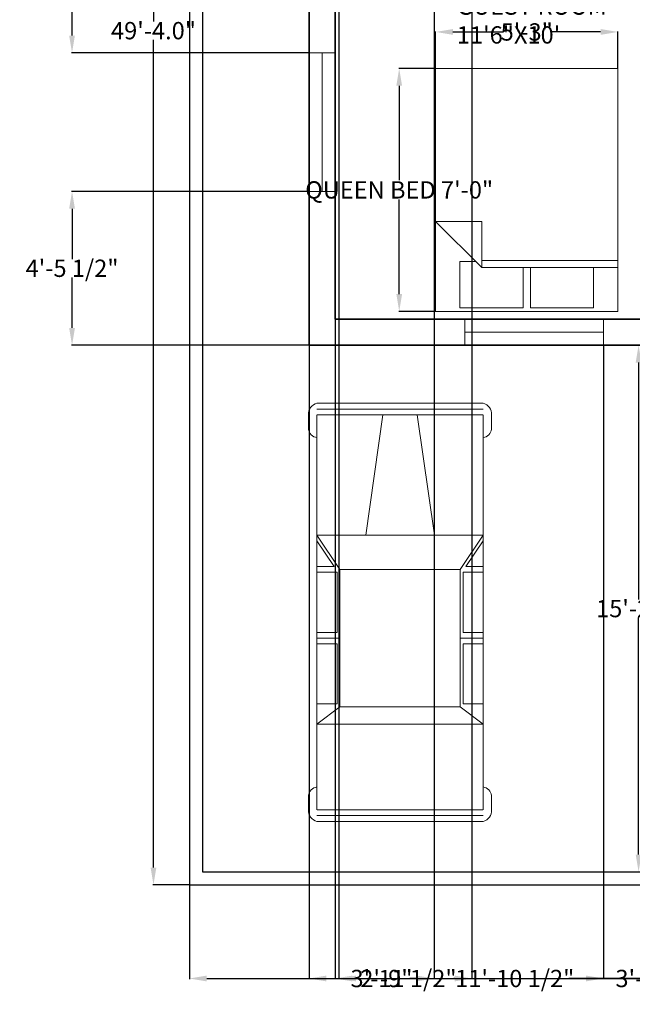
# Model space of a CAD drawing. Units: inches. Extents: x 889 to 1449, y 3224 to 3899.
# Tile 1 of 4: x 889 to 1101, y 3224 to 3565. Entities that reach past the tile are written whole.
import ezdxf

# ---------------------------------------------------------------- set-up
doc = ezdxf.new("R2010")
doc.units = ezdxf.units.IN
doc.header["$MEASUREMENT"] = 0
for name, color, linetype, lineweight in [('A-ANNO-DIMS', 2, 'Continuous', 18), ('A-AREA-IDEN', 7, 'Continuous', 18), ('A-FURN', 8, 'Continuous', 18), ('A-GLAZ', 4, 'Continuous', 18), ('A-WALL', 7, 'Continuous', 35), ('C-PROP', 7, 'Continuous', 25), ('C-SITE-VEHC', 8, 'Continuous', 18)]:
    doc.layers.add(name, color=color, linetype=linetype, lineweight=lineweight)
doc.styles.get("Standard").update_dxf_attribs({"font": 'arial.ttf'})
doc.dimstyles.get("Standard").update_dxf_attribs({"dimtxt": 6, "dimasz": 6, "dimexe": 0.18, "dimexo": 0.0625, "dimgap": 0.09, "dimtad": 0, "dimtih": 1, "dimtoh": 1, "dimdec": 1, "dimzin": 0, "dimdsep": 46, "dimlunit": 3, "dimtxsty": 'Standard', "dimcen": 0.09, "dimadec": 0, "dimazin": 0, "dimtfac": 1, "dimtdec": 1, "dimtofl": 0, "dimtmove": 0, "dimatfit": 3, "dimfxl": 1, "dimtolj": 1, "dimtzin": 0, "dimarcsym": 0})

# ---------------------------------------------------------------- blocks, each defined once
blk = doc.blocks.new('*U13')
for p, q in [((5.44, 42.31), (12.12, 42.31)), ((189.69, 42.31), (183.01, 42.31)), ((0.1, -0.41), (0.1, 38.35)), ((2.77, -0.41), (2.77, 38.31)), ((5.44, -0.41), (5.44, 38.24)), ((5.45, 38.31), (16.12, 38.31)), ((16.12, 38.31), (180.34, 38.31)), ((61.52, -0.41), (61.52, 38.31)), ((61.52, 38.31), (77.54, 27.62)), ((64.19, 38.31), (76.2, 30.29)), ((76.2, 30.29), (76.2, 38.31)), ((78.87, 38.31), (78.87, 28.96)), ((106.91, 28.96), (106.91, 38.31)), ((109.58, 27.62), (109.58, 38.31)), ((112.25, 38.31), (112.25, 28.96)), ((140.29, 28.96), (140.29, 38.31)), ((141.62, 27.62), (149.64, 38.31)), ((149.64, -0.41), (149.64, 38.31)), ((189.69, 38.31), (179.01, 38.31)), ((189.69, -0.41), (189.69, 38.24)), ((192.36, -0.41), (192.36, 38.31)), ((195.03, -0.41), (195.03, 38.35)), ((77.54, 27.62), (141.62, 27.62)), ((77.54, -0.41), (77.54, 27.62)), ((78.87, 28.96), (106.91, 28.96)), ((112.25, 28.96), (140.29, 28.96)), ((141.62, -0.41), (141.62, 27.62)), ((5.44, 7.6), (61.52, 15.61)), ((0.1, -0.42), (0.1, -39.18)), ((2.77, -0.41), (2.77, -39.13)), ((5.44, -0.42), (5.44, -39.07)), ((61.52, -0.41), (61.52, -39.13)), ((77.54, -0.41), (77.54, -28.45)), ((141.62, -0.41), (141.62, -28.45)), ((149.64, -0.41), (149.64, -39.13)), ((189.69, -0.42), (189.69, -39.07)), ((192.36, -0.41), (192.36, -39.13)), ((195.03, -0.42), (195.03, -39.18)), ((5.44, -8.42), (61.52, -16.43)), ((61.52, -39.13), (77.54, -28.45)), ((64.19, -39.13), (76.2, -31.12)), ((76.2, -31.12), (76.2, -39.13)), ((77.54, -28.45), (141.62, -28.45)), ((78.87, -39.13), (78.87, -29.79)), ((78.87, -29.79), (106.91, -29.79)), ((106.91, -29.79), (106.91, -39.13)), ((109.58, -28.45), (109.58, -39.13)), ((112.25, -29.79), (140.29, -29.79)), ((112.25, -39.13), (112.25, -29.79)), ((140.29, -29.79), (140.29, -39.13)), ((141.62, -28.45), (149.64, -39.13)), ((5.45, -39.13), (16.12, -39.13)), ((16.12, -39.13), (180.34, -39.13)), ((189.69, -39.13), (179.01, -39.13)), ((5.44, -43.14), (12.12, -43.14)), ((189.69, -43.14), (183.01, -43.14))]:
    blk.add_line(p, q)
for centre, radius, start, end in [((5.06, 37.26), 5.06, 85.6455, 168.0943), ((11.45, 37.64), 4.72, 8.1301, 81.87), ((183.68, 37.64), 4.72, 98.13, 171.8699), ((190.07, 37.26), 5.06, 11.9057, 94.3545), ((5.06, -38.09), 5.06, 191.9057, 274.3545), ((11.45, -38.46), 4.72, 278.13, 351.8699), ((183.68, -38.46), 4.72, 188.1301, 261.87), ((190.07, -38.09), 5.06, 265.6455, 348.0943)]:
    blk.add_arc(centre, radius, start, end)
blk = doc.blocks.new('Bed - Queen')
for p, q in [((0, -80.00003), (0, 0)), ((0, 0), (59.99999, 0)), ((59.99999, 0), (59.99999, -80.00003)), ((7.99999, -1.2), (28.79998, -1.2)), ((7.99999, -14.4), (7.99999, -1.2)), ((28.79998, -1.2), (28.79998, -14.4)), ((31.19999, -1.2), (51.99999, -1.2)), ((31.19999, -14.4), (31.19999, -1.2)), ((51.99999, -1.2), (51.99999, -16.4)), ((0, -14.4), (44.8, -14.4)), ((59.99999, -29.6), (44.8, -14.4)), ((44.8, -14.4), (44.8, -29.6)), ((44.8, -16.8), (0, -16.8)), ((51.99999, -16.4), (46.79936, -16.4)), ((44.8, -29.6), (59.99999, -29.6)), ((59.99999, -80.00003), (0, -80.00003))]:
    blk.add_line(p, q)
blk = doc.blocks.new('*D19')
at = {"layer": 'A-ANNO-DIMS', "color": 0, "lineweight": -2, "transparency": 16777216}
for p, q in [((947.88, 3857.35), (935.33, 3857.35)), ((935.51, 3851.35), (935.51, 3564.51)), ((935.51, 3271.35), (935.51, 3558.2)), ((947.88, 3265.35), (935.33, 3265.35))]:
    blk.add_line(p, q, dxfattribs=at)
at = {"layer": 'A-ANNO-DIMS', "color": 0, "transparency": 16777216}
for points in [[(934.51, 3851.35), (936.51, 3851.35), (935.51, 3857.35)], [(934.51, 3271.35), (936.51, 3271.35), (935.51, 3265.35)]]:
    blk.add_solid(points, dxfattribs=at)
at = {"layer": 'Defpoints', "color": 0, "transparency": 16777216}
for p in [(947.95, 3857.35), (935.51, 3265.35), (947.95, 3265.35)]:
    blk.add_point(p, dxfattribs=at)
at = {"layer": 'A-ANNO-DIMS', "color": 0, "transparency": 16777216, "insert": (935.51, 3561.35), "char_height": 6, "attachment_point": 5}
blk.add_mtext('\\A1;49\'-4.0"', dxfattribs=at)
blk = doc.blocks.new('*D22')
at = {"layer": 'A-ANNO-DIMS', "color": 0, "lineweight": -2, "transparency": 16777216}
for p, q in [((1103.67, 3452.35), (1103.79, 3452.35)), ((1103.61, 3446.35), (1103.61, 3364.26)), ((1103.61, 3275.85), (1103.61, 3357.95)), ((1103.67, 3269.85), (1103.79, 3269.85))]:
    blk.add_line(p, q, dxfattribs=at)
at = {"layer": 'A-ANNO-DIMS', "color": 0, "transparency": 16777216}
for points in [[(1102.61, 3446.35), (1104.61, 3446.35), (1103.61, 3452.35)], [(1102.61, 3275.85), (1104.61, 3275.85), (1103.61, 3269.85)]]:
    blk.add_solid(points, dxfattribs=at)
at = {"layer": 'Defpoints', "color": 0, "transparency": 16777216}
for p in [(1103.61, 3452.35), (1103.61, 3269.85), (1103.61, 3269.85)]:
    blk.add_point(p, dxfattribs=at)
at = {"layer": 'A-ANNO-DIMS', "color": 0, "transparency": 16777216, "insert": (1103.61, 3361.1), "char_height": 6, "attachment_point": 5}
blk.add_mtext('\\A1;15\'-2.5"', dxfattribs=at)
blk = doc.blocks.new('WIN-48IN')
blk.add_line((4.5, 48), (4.5, 0))
blk.add_lwpolyline([(9, 48), (9, 0), (0, 0), (0, 48)], close=True)
blk = doc.blocks.new('*D32')
at = {"layer": 'A-ANNO-DIMS', "color": 0, "lineweight": -2, "transparency": 16777216}
for p, q in [((1033.22, 3548.27), (1020.48, 3548.27)), ((1020.66, 3542.27), (1020.66, 3509.55)), ((1020.66, 3470.08), (1020.66, 3502.8)), ((1033.22, 3464.08), (1020.48, 3464.08))]:
    blk.add_line(p, q, dxfattribs=at)
at = {"layer": 'A-ANNO-DIMS', "color": 0, "transparency": 16777216}
for points in [[(1019.66, 3542.27), (1021.66, 3542.27), (1020.66, 3548.27)], [(1019.66, 3470.08), (1021.66, 3470.08), (1020.66, 3464.08)]]:
    blk.add_solid(points, dxfattribs=at)
at = {"layer": 'Defpoints', "color": 0, "transparency": 16777216}
for p in [(1033.28, 3548.27), (1020.66, 3464.08), (1033.28, 3464.08)]:
    blk.add_point(p, dxfattribs=at)
at = {"layer": 'A-ANNO-DIMS', "color": 0, "transparency": 16777216, "insert": (1020.66, 3506.17), "char_height": 6, "attachment_point": 5}
blk.add_mtext('\\A1;QUEEN BED 7\'-0"', dxfattribs=at)
blk = doc.blocks.new('*D33')
at = {"layer": 'A-ANNO-DIMS', "color": 0, "lineweight": -2, "transparency": 16777216}
for p, q in [((1033.28, 3548.34), (1033.28, 3561.08)), ((1039.28, 3560.9), (1056.79, 3560.9)), ((1090.43, 3560.9), (1072.92, 3560.9)), ((1096.43, 3548.34), (1096.43, 3561.08))]:
    blk.add_line(p, q, dxfattribs=at)
at = {"layer": 'A-ANNO-DIMS', "color": 0, "transparency": 16777216}
for points in [[(1039.28, 3561.9), (1039.28, 3559.9), (1033.28, 3560.9)], [(1090.43, 3561.9), (1090.43, 3559.9), (1096.43, 3560.9)]]:
    blk.add_solid(points, dxfattribs=at)
at = {"layer": 'Defpoints', "color": 0, "transparency": 16777216}
for p in [(1033.28, 3560.9), (1033.28, 3548.27), (1096.43, 3548.27)]:
    blk.add_point(p, dxfattribs=at)
at = {"layer": 'A-ANNO-DIMS', "color": 0, "transparency": 16777216, "insert": (1064.86, 3560.9), "char_height": 6, "attachment_point": 5}
blk.add_mtext('\\A1;5\'-3"', dxfattribs=at)
blk = doc.blocks.new('*D44')
at = {"layer": 'A-ANNO-DIMS', "color": 0, "lineweight": -2, "transparency": 16777216}
for p, q in [((947.95, 3265.29), (947.95, 3232.74)), ((1400.45, 3265.29), (1400.45, 3232.74)), ((953.95, 3232.92), (1156.81, 3232.92)), ((1394.45, 3232.92), (1191.58, 3232.92))]:
    blk.add_line(p, q, dxfattribs=at)
at = {"layer": 'A-ANNO-DIMS', "color": 0, "transparency": 16777216}
for points in [[(953.95, 3233.92), (953.95, 3231.92), (947.95, 3232.92)], [(1394.45, 3233.92), (1394.45, 3231.92), (1400.45, 3232.92)]]:
    blk.add_solid(points, dxfattribs=at)
at = {"layer": 'Defpoints', "color": 0, "transparency": 16777216}
for p in [(947.95, 3265.35), (1400.45, 3265.35), (1400.45, 3232.92)]:
    blk.add_point(p, dxfattribs=at)
at = {"layer": 'A-ANNO-DIMS', "color": 0, "transparency": 16777216, "insert": (1174.2, 3232.92), "char_height": 6, "attachment_point": 5}
blk.add_mtext('\\A1;37\'-8 1/2"', dxfattribs=at)
blk = doc.blocks.new('*D48')
at = {"layer": 'A-ANNO-DIMS', "color": 0, "lineweight": -2, "transparency": 16777216}
for p, q in [((989.45, 3452.29), (989.45, 3232.74)), ((1131.95, 3452.29), (1131.95, 3232.74)), ((995.45, 3232.92), (1041.26, 3232.92)), ((1125.95, 3232.92), (1080.13, 3232.92))]:
    blk.add_line(p, q, dxfattribs=at)
at = {"layer": 'A-ANNO-DIMS', "color": 0, "transparency": 16777216}
for points in [[(995.45, 3233.92), (995.45, 3231.92), (989.45, 3232.92)], [(1125.95, 3233.92), (1125.95, 3231.92), (1131.95, 3232.92)]]:
    blk.add_solid(points, dxfattribs=at)
at = {"layer": 'Defpoints', "color": 0, "transparency": 16777216}
for p in [(989.45, 3452.35), (1131.95, 3452.35), (1131.95, 3232.92)]:
    blk.add_point(p, dxfattribs=at)
at = {"layer": 'A-ANNO-DIMS', "color": 0, "transparency": 16777216, "insert": (1060.7, 3232.92), "char_height": 6, "attachment_point": 5}
blk.add_mtext('\\A1;11\'-10 1/2"', dxfattribs=at)
blk = doc.blocks.new('*D52')
at = {"layer": 'A-ANNO-DIMS', "color": 0, "lineweight": -2, "transparency": 16777216}
for p, q in [((989.38, 3505.66), (907.11, 3505.66)), ((907.29, 3499.66), (907.29, 3482.2)), ((907.29, 3458.35), (907.29, 3475.82)), ((989.38, 3452.35), (907.11, 3452.35))]:
    blk.add_line(p, q, dxfattribs=at)
at = {"layer": 'A-ANNO-DIMS', "color": 0, "transparency": 16777216}
for points in [[(906.29, 3499.66), (908.29, 3499.66), (907.29, 3505.66)], [(906.29, 3458.35), (908.29, 3458.35), (907.29, 3452.35)]]:
    blk.add_solid(points, dxfattribs=at)
at = {"layer": 'Defpoints', "color": 0, "transparency": 16777216}
for p in [(907.29, 3505.66), (989.45, 3505.66), (989.45, 3452.35)]:
    blk.add_point(p, dxfattribs=at)
at = {"layer": 'A-ANNO-DIMS', "color": 0, "transparency": 16777216, "insert": (907.29, 3479.01), "char_height": 6, "attachment_point": 5}
blk.add_mtext('\\A1;4\'-5 1/2"', dxfattribs=at)
blk = doc.blocks.new('*D53')
at = {"layer": 'A-ANNO-DIMS', "color": 0, "lineweight": -2, "transparency": 16777216}
for p, q in [((989.38, 3600.04), (907.11, 3600.04)), ((907.29, 3594.04), (907.29, 3580.05)), ((907.29, 3559.66), (907.29, 3573.66)), ((989.38, 3553.66), (907.11, 3553.66))]:
    blk.add_line(p, q, dxfattribs=at)
at = {"layer": 'A-ANNO-DIMS', "color": 0, "transparency": 16777216}
for points in [[(906.29, 3594.04), (908.29, 3594.04), (907.29, 3600.04)], [(906.29, 3559.66), (908.29, 3559.66), (907.29, 3553.66)]]:
    blk.add_solid(points, dxfattribs=at)
at = {"layer": 'Defpoints', "color": 0, "transparency": 16777216}
for p in [(907.29, 3600.04), (989.45, 3600.04), (989.45, 3553.66)]:
    blk.add_point(p, dxfattribs=at)
at = {"layer": 'A-ANNO-DIMS', "color": 0, "transparency": 16777216, "insert": (907.29, 3576.85), "char_height": 6, "attachment_point": 5}
blk.add_mtext('\\A1;3\'-10 1/2"', dxfattribs=at)
blk = doc.blocks.new('*D57')
at = {"layer": 'A-ANNO-DIMS', "color": 0, "lineweight": -2, "transparency": 16777216}
for p, q in [((1091.445734, 3452.292373), (1091.445734, 3232.744873)), ((1131.945734, 3452.292373), (1131.945734, 3232.744873)), ((1085.445734, 3232.924873), (1079.445734, 3232.924873)), ((1137.945734, 3232.924873), (1143.945734, 3232.924873))]:
    blk.add_line(p, q, dxfattribs=at)
at = {"layer": 'A-ANNO-DIMS', "color": 0, "transparency": 16777216}
for points in [[(1085.445734, 3233.924873), (1085.445734, 3231.924873), (1091.445734, 3232.924873)], [(1137.945734, 3233.924873), (1137.945734, 3231.924873), (1131.945734, 3232.924873)]]:
    blk.add_solid(points, dxfattribs=at)
at = {"layer": 'Defpoints', "color": 0, "transparency": 16777216}
for p in [(1091.445734, 3452.354873), (1131.945734, 3452.354873), (1131.945734, 3232.924873)]:
    blk.add_point(p, dxfattribs=at)
at = {"layer": 'A-ANNO-DIMS', "color": 0, "transparency": 16777216, "insert": (1111.695734, 3232.924873), "char_height": 6, "attachment_point": 5}
blk.add_mtext('\\A1;3\'-4 1/2"', dxfattribs=at)
blk = doc.blocks.new('*D62')
at = {"layer": 'A-ANNO-DIMS', "color": 0, "lineweight": -2, "transparency": 16777216}
for p, q in [((998.45, 3710.29), (998.45, 3232.74)), ((1045.87, 3710.29), (1045.87, 3232.74)), ((1004.45, 3232.92), (1004.77, 3232.92)), ((1039.87, 3232.92), (1039.54, 3232.92))]:
    blk.add_line(p, q, dxfattribs=at)
at = {"layer": 'A-ANNO-DIMS', "color": 0, "transparency": 16777216}
for points in [[(1004.45, 3233.92), (1004.45, 3231.92), (998.45, 3232.92)], [(1039.87, 3233.92), (1039.87, 3231.92), (1045.87, 3232.92)]]:
    blk.add_solid(points, dxfattribs=at)
at = {"layer": 'Defpoints', "color": 0, "transparency": 16777216}
for p in [(998.45, 3710.35), (1045.87, 3710.35), (1045.87, 3232.92)]:
    blk.add_point(p, dxfattribs=at)
at = {"layer": 'A-ANNO-DIMS', "color": 0, "transparency": 16777216, "insert": (1022.16, 3232.92), "char_height": 6, "attachment_point": 5}
blk.add_mtext('\\A1;3\'-11 1/2"', dxfattribs=at)
blk = doc.blocks.new('*D63')
at = {"layer": 'A-ANNO-DIMS', "color": 0, "lineweight": -2, "transparency": 16777216}
for p, q in [((999.72, 3690.79), (999.72, 3232.74)), ((1032.72, 3680.29), (1032.72, 3232.74)), ((1005.72, 3232.92), (1008.1, 3232.92)), ((1026.72, 3232.92), (1024.33, 3232.92))]:
    blk.add_line(p, q, dxfattribs=at)
at = {"layer": 'A-ANNO-DIMS', "color": 0, "transparency": 16777216}
for points in [[(1005.72, 3233.92), (1005.72, 3231.92), (999.72, 3232.92)], [(1026.72, 3233.92), (1026.72, 3231.92), (1032.72, 3232.92)]]:
    blk.add_solid(points, dxfattribs=at)
at = {"layer": 'Defpoints', "color": 0, "transparency": 16777216}
for p in [(999.72, 3690.85), (1032.72, 3680.35), (1032.72, 3232.92)]:
    blk.add_point(p, dxfattribs=at)
at = {"layer": 'A-ANNO-DIMS', "color": 0, "transparency": 16777216, "insert": (1016.22, 3232.92), "char_height": 6, "attachment_point": 5}
blk.add_mtext('\\A1;2\'-9"', dxfattribs=at)

msp = doc.modelspace()

# ---------------------------------------------------------------- linework, layer by layer
at = {"layer": 'A-WALL'}
for p, q in [((989.45, 3852.85), (989.45, 3452.35)), ((998.45, 3645.85), (998.45, 3461.35)), ((998.45, 3461.35), (1136.45, 3461.35)), ((989.45, 3452.35), (1131.95, 3452.35))]:
    msp.add_line(p, q, dxfattribs=at)
at = {"layer": 'C-PROP'}
for p, q in [((947.95, 3857.35), (947.95, 3265.35)), ((952.45, 3852.85), (952.45, 3269.85)), ((952.45, 3269.85), (1395.95, 3269.85)), ((947.95, 3265.35), (1400.45, 3265.35))]:
    msp.add_line(p, q, dxfattribs=at)

# ---------------------------------------------------------------- block references
at = {"layer": 'A-FURN', "xscale": 1.052472781090682, "yscale": 1.052472781090682, "zscale": 1.052472781090682, "rotation": 180}
msp.add_blockref('Bed - Queen', (1096.43, 3464.08), dxfattribs=at)
at = {"layer": 'A-GLAZ'}
msp.add_blockref('WIN-48IN', (989.45, 3505.66), dxfattribs=at)
at = {"layer": 'A-GLAZ', "rotation": 90.00000000000063}
msp.add_blockref('WIN-48IN', (1091.45, 3452.36), dxfattribs=at)
at = {"layer": 'C-SITE-VEHC', "xscale": 0.7431121198183446, "yscale": 0.7431121198183446, "zscale": 0.7431121198183446, "rotation": 270}
msp.add_blockref('*U13', (1021.25, 3432.3), dxfattribs=at)

# ---------------------------------------------------------------- texts
at = {"layer": 'A-AREA-IDEN', "insert": (1040.64, 3572.87), "char_height": 6, "attachment_point": 1}
msp.add_mtext_dynamic_manual_height_columns('GUEST ROOM\\P11\'6"X10\'', width=93.4406, gutter_width=1, heights=[0], dxfattribs=at)

# ---------------------------------------------------------------- dimensions: what is measured, and where the dimension line sits
at = {"layer": 'A-ANNO-DIMS'}
for base, p1, p2, angle, override, picture, middle in [((935.51, 3265.35), (947.95, 3857.35), (947.95, 3265.35), 90, {"dimclrd": 0, "dimclre": 0, "dimclrt": 0}, '*D19', (935.51, 3561.35)), ((907.29, 3600.04), (989.45, 3553.66), (989.45, 3600.04), 90, {"dimdec": 1, "dimlfac": 1, "dimrnd": 0, "dimzin": 1, "dimdsep": 46, "dimlunit": 4, "dimfrac": 2}, '*D53', (907.29, 3576.85)), ((1033.2849, 3560.903), (1096.4332, 3548.2733), (1033.2849, 3548.2733), 180, {"dimdec": 1, "dimlfac": 1, "dimrnd": 0, "dimzin": 1, "dimdsep": 46, "dimlunit": 4, "dimfrac": 2}, '*D33', (1064.859, 3560.903)), ((907.29, 3505.66), (989.45, 3452.35), (989.45, 3505.66), 90, {"dimdec": 1, "dimlfac": 1, "dimrnd": 0, "dimzin": 1, "dimdsep": 46, "dimlunit": 4, "dimfrac": 2}, '*D52', (907.29, 3479.01)), ((1103.61, 3269.85), (1103.61, 3452.35), (1103.61, 3269.85), 90, {"dimclrd": 0, "dimclre": 0, "dimclrt": 0}, '*D22', (1103.61, 3361.1))]:
    dim = msp.add_linear_dim(base=base, p1=p1, p2=p2, angle=angle, dimstyle='Standard', override=override, dxfattribs=at)
    dim.commit()
    dim.dimension.update_dxf_attribs({"geometry": picture, "text_midpoint": middle})
for base, p1, p2, picture, middle in [((1045.87, 3232.92), (998.45, 3710.35), (1045.87, 3710.35), '*D62', (1022.16, 3232.92)), ((1032.72, 3232.92), (999.72, 3690.85), (1032.72, 3680.35), '*D63', (1016.22, 3232.92)), ((1131.95, 3232.92), (989.45, 3452.35), (1131.95, 3452.35), '*D48', (1060.7, 3232.92)), ((1131.95, 3232.92), (1091.45, 3452.35), (1131.95, 3452.35), '*D57', (1111.7, 3232.92)), ((1400.45, 3232.92), (947.95, 3265.35), (1400.45, 3265.35), '*D44', (1174.2, 3232.92))]:
    dim = msp.add_linear_dim(base=base, p1=p1, p2=p2, dimstyle='Standard', override={"dimdec": 1, "dimlfac": 1, "dimrnd": 0, "dimzin": 1, "dimdsep": 46, "dimlunit": 4, "dimfrac": 2}, dxfattribs=at)
    dim.commit()
    dim.dimension.update_dxf_attribs({"geometry": picture, "text_midpoint": middle})
dim = msp.add_linear_dim(base=(1020.66, 3464.08), p1=(1033.28, 3548.27), p2=(1033.28, 3464.08), angle=270, text='QUEEN BED <>', dimstyle='Standard', override={"dimdec": 1, "dimlfac": 1, "dimrnd": 0, "dimzin": 1, "dimdsep": 46, "dimlunit": 4, "dimfrac": 2}, dxfattribs=at)
dim.commit()
dim.dimension.update_dxf_attribs({"geometry": '*D32', "text_midpoint": (1020.66, 3506.17)})

doc.saveas('drawing.dxf')
